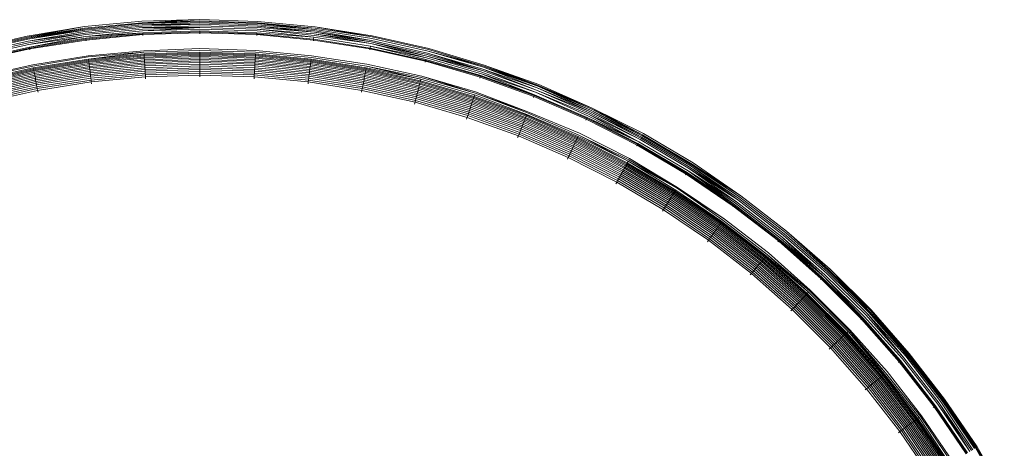
# Model space of a CAD drawing. Units: inches. Extents: x 64 to 1167, y 117 to 939.
# Tile 54 of 56: x 1130.034 to 1131.241, y 501.546 to 502.071. Entities that reach past the tile are written whole.
import ezdxf

# ---------------------------------------------------------------- set-up
doc = ezdxf.new("R2010")
doc.units = ezdxf.units.IN
doc.header["$MEASUREMENT"] = 0
doc.layers.add('A-FLOR-FIXT', color=8, linetype='Continuous', lineweight=18)

msp = doc.modelspace()

# ---------------------------------------------------------------- linework, layer by layer
at = {"layer": 'A-FLOR-FIXT'}
for p, q in [((1130.1137, 502.0626), (1130.0437, 502.0509)), ((1130.1137, 502.0626), (1130.044, 502.0497)), ((1130.1843, 502.0693), (1130.1137, 502.0626)), ((1130.1844, 502.0675), (1130.1139, 502.0608)), ((1130.1845, 502.0663), (1130.114, 502.0596)), ((1130.1845, 502.0649), (1130.1142, 502.0583)), ((1130.1847, 502.0633), (1130.1144, 502.0566)), ((1130.2552, 502.0712), (1130.1843, 502.0693)), ((1130.2552, 502.0712), (1130.1844, 502.0675)), ((1130.2552, 502.0697), (1130.1844, 502.0675)), ((1130.2552, 502.0685), (1130.1844, 502.0675)), ((1130.2552, 502.0685), (1130.1845, 502.0663)), ((1130.2552, 502.0671), (1130.1845, 502.0649)), ((1130.2552, 502.0655), (1130.1845, 502.0649)), ((1130.2552, 502.0655), (1130.1847, 502.0633)), ((1130.2552, 502.0637), (1130.1848, 502.0614)), ((1130.326, 502.0689), (1130.2552, 502.0712)), ((1130.3259, 502.0675), (1130.2552, 502.0697)), ((1130.3258, 502.0663), (1130.2552, 502.0685)), ((1130.3258, 502.0649), (1130.2552, 502.0671)), ((1130.3257, 502.0633), (1130.2552, 502.0655)), ((1130.3255, 502.0614), (1130.2552, 502.0637)), ((1130.396, 502.0575), (1130.3257, 502.0633)), ((1130.3958, 502.0558), (1130.3257, 502.0633)), ((1130.3962, 502.059), (1130.3258, 502.0663)), ((1130.3964, 502.0608), (1130.3258, 502.0663)), ((1130.3962, 502.059), (1130.3258, 502.0649)), ((1130.3964, 502.0608), (1130.3259, 502.0675)), ((1130.3966, 502.0623), (1130.326, 502.0689)), ((1130.0437, 502.0509), (1129.9746, 502.0355)), ((1130.1139, 502.0608), (1130.044, 502.0497)), ((1130.1139, 502.0608), (1130.0442, 502.0486)), ((1130.114, 502.0596), (1130.0442, 502.0486)), ((1130.1142, 502.0583), (1130.0442, 502.0486)), ((1130.1142, 502.0583), (1130.0445, 502.0472)), ((1130.1144, 502.0566), (1130.0449, 502.0447)), ((1130.1147, 502.0548), (1130.0449, 502.0447)), ((1130.1147, 502.0548), (1130.0453, 502.0428)), ((1130.1149, 502.0528), (1130.0457, 502.0408)), ((1130.1152, 502.0507), (1130.0457, 502.0408)), ((1130.1152, 502.0507), (1130.0463, 502.0376)), ((1130.1848, 502.0614), (1130.1147, 502.0548)), ((1130.1849, 502.0595), (1130.1149, 502.0528)), ((1130.185, 502.0573), (1130.1152, 502.0507)), ((1130.1852, 502.0551), (1130.1152, 502.0507)), ((1130.1852, 502.0551), (1130.1155, 502.0485)), ((1130.1852, 502.054), (1130.1156, 502.0474)), ((1130.1853, 502.0528), (1130.1157, 502.0462)), ((1130.2552, 502.0617), (1130.1848, 502.0614)), ((1130.2552, 502.0617), (1130.1849, 502.0595)), ((1130.2552, 502.0617), (1130.185, 502.0573)), ((1130.2552, 502.0595), (1130.185, 502.0573)), ((1130.2552, 502.0573), (1130.1852, 502.0551)), ((1130.2552, 502.0562), (1130.1852, 502.054)), ((1130.1852, 502.054), (1130.1852, 502.0551)), ((1130.1853, 502.0528), (1130.1852, 502.054)), ((1130.2552, 502.055), (1130.1853, 502.0528)), ((1130.1854, 502.0517), (1130.1853, 502.0528)), ((1130.3254, 502.0595), (1130.2552, 502.0617)), ((1130.3253, 502.0573), (1130.2552, 502.0595)), ((1130.3251, 502.0551), (1130.2552, 502.0573)), ((1130.2552, 502.0573), (1130.2552, 502.0562)), ((1130.3251, 502.054), (1130.2552, 502.0562)), ((1130.2552, 502.0562), (1130.2552, 502.055)), ((1130.325, 502.0528), (1130.2552, 502.055)), ((1130.2552, 502.055), (1130.2552, 502.0539)), ((1130.325, 502.0528), (1130.3249, 502.0517)), ((1130.3251, 502.054), (1130.325, 502.0528)), ((1130.3946, 502.0462), (1130.325, 502.0528)), ((1130.3251, 502.0551), (1130.3251, 502.054)), ((1130.395, 502.0496), (1130.3251, 502.0551)), ((1130.3947, 502.0474), (1130.3251, 502.054)), ((1130.395, 502.0496), (1130.3253, 502.0573)), ((1130.3955, 502.0538), (1130.3254, 502.0595)), ((1130.3953, 502.0518), (1130.3254, 502.0595)), ((1130.3958, 502.0558), (1130.3255, 502.0614)), ((1130.4648, 502.0418), (1130.3953, 502.0518)), ((1130.4648, 502.0418), (1130.3955, 502.0538)), ((1130.4652, 502.0438), (1130.3955, 502.0538)), ((1130.4655, 502.0456), (1130.3958, 502.0558)), ((1130.4652, 502.0438), (1130.3958, 502.0558)), ((1130.4655, 502.0456), (1130.396, 502.0575)), ((1130.466, 502.0479), (1130.3962, 502.059)), ((1130.4664, 502.0502), (1130.3964, 502.0608)), ((1130.4666, 502.0514), (1130.3966, 502.0623)), ((1130.4664, 502.0502), (1130.3966, 502.0623)), ((1130.5358, 502.0359), (1130.4666, 502.0514)), ((1130.044, 502.0497), (1129.9749, 502.0343)), ((1130.0442, 502.0486), (1129.9752, 502.0332)), ((1130.0445, 502.0472), (1129.9755, 502.0318)), ((1130.0449, 502.0447), (1129.9761, 502.0294)), ((1130.0453, 502.0428), (1129.9766, 502.0275)), ((1130.0457, 502.0408), (1129.9771, 502.0255)), ((1130.1155, 502.0485), (1130.0463, 502.0376)), ((1130.1156, 502.0474), (1130.0465, 502.0364)), ((1130.1157, 502.0462), (1130.0467, 502.0353)), ((1130.1156, 502.0474), (1130.1155, 502.0485)), ((1130.1157, 502.0462), (1130.1156, 502.0474)), ((1130.1159, 502.0451), (1130.1157, 502.0462)), ((1130.3944, 502.0451), (1130.3946, 502.0462)), ((1130.3946, 502.0462), (1130.3947, 502.0474)), ((1130.4636, 502.0353), (1130.3946, 502.0462)), ((1130.3947, 502.0474), (1130.395, 502.0496)), ((1130.4638, 502.0364), (1130.3947, 502.0474)), ((1130.4642, 502.0387), (1130.395, 502.0496)), ((1130.4642, 502.0387), (1130.4638, 502.0364)), ((1130.5329, 502.0244), (1130.4642, 502.0387)), ((1130.5323, 502.0223), (1130.4642, 502.0387)), ((1130.5329, 502.0244), (1130.4648, 502.0418)), ((1130.5334, 502.0265), (1130.4648, 502.0418)), ((1130.5339, 502.0284), (1130.4652, 502.0438)), ((1130.5334, 502.0265), (1130.4652, 502.0438)), ((1130.5344, 502.0302), (1130.4655, 502.0456)), ((1130.535, 502.0325), (1130.466, 502.0479)), ((1130.5355, 502.0347), (1130.4664, 502.0502)), ((1130.0463, 502.0376), (1129.978, 502.0223)), ((1130.0465, 502.0364), (1129.9782, 502.0212)), ((1130.0467, 502.0353), (1129.9785, 502.0201)), ((1130.0463, 502.0376), (1130.0465, 502.0364)), ((1130.0465, 502.0364), (1130.0467, 502.0353)), ((1130.0467, 502.0353), (1130.0469, 502.0342)), ((1130.1182, 502.0269), (1130.0505, 502.0157)), ((1130.1866, 502.0329), (1130.1182, 502.0269)), ((1130.1867, 502.0314), (1130.1183, 502.0257)), ((1130.1867, 502.0314), (1130.1187, 502.0229)), ((1130.1868, 502.0293), (1130.1187, 502.0229)), ((1130.1869, 502.0281), (1130.1188, 502.0217)), ((1130.1869, 502.0268), (1130.119, 502.0204)), ((1130.2552, 502.0359), (1130.1866, 502.0329)), ((1130.2552, 502.0335), (1130.1867, 502.0314)), ((1130.2552, 502.0315), (1130.1868, 502.0293)), ((1130.1869, 502.0281), (1130.1868, 502.0293)), ((1130.2552, 502.0303), (1130.1869, 502.0281)), ((1130.2552, 502.0289), (1130.1869, 502.0268)), ((1130.1869, 502.0268), (1130.1869, 502.0281)), ((1130.187, 502.0253), (1130.1869, 502.0268)), ((1130.2552, 502.0275), (1130.187, 502.0253)), ((1130.3238, 502.0334), (1130.2552, 502.0359)), ((1130.3236, 502.0314), (1130.2552, 502.0335)), ((1130.3235, 502.0293), (1130.2552, 502.0315)), ((1130.2552, 502.0303), (1130.2552, 502.0315)), ((1130.3234, 502.0281), (1130.2552, 502.0303)), ((1130.2552, 502.0289), (1130.2552, 502.0303)), ((1130.3234, 502.0268), (1130.2552, 502.0289)), ((1130.2552, 502.0275), (1130.2552, 502.0289)), ((1130.3233, 502.0253), (1130.2552, 502.0275)), ((1130.2552, 502.0259), (1130.2552, 502.0275)), ((1130.3233, 502.0253), (1130.3234, 502.0268)), ((1130.3234, 502.0281), (1130.3235, 502.0293)), ((1130.3915, 502.0217), (1130.3234, 502.0281)), ((1130.3234, 502.0268), (1130.3234, 502.0281)), ((1130.3913, 502.0204), (1130.3234, 502.0268)), ((1130.3916, 502.0229), (1130.3235, 502.0293)), ((1130.3919, 502.0249), (1130.3236, 502.0314)), ((1130.3921, 502.0269), (1130.3238, 502.0334)), ((1130.46, 502.0168), (1130.3921, 502.0269)), ((1130.4636, 502.0353), (1130.4634, 502.0342)), ((1130.4638, 502.0364), (1130.4636, 502.0353)), ((1130.5318, 502.0201), (1130.4636, 502.0353)), ((1130.5321, 502.0212), (1130.4638, 502.0364)), ((1130.6009, 502.0069), (1130.5334, 502.0265)), ((1130.6015, 502.0088), (1130.5334, 502.0265)), ((1130.6015, 502.0088), (1130.5339, 502.0284)), ((1130.6015, 502.0088), (1130.5344, 502.0302)), ((1130.6021, 502.0105), (1130.5344, 502.0302)), ((1130.6028, 502.0128), (1130.535, 502.0325)), ((1130.6032, 502.014), (1130.535, 502.0325)), ((1130.6032, 502.014), (1130.5355, 502.0347)), ((1130.6037, 502.0154), (1130.5358, 502.0359)), ((1130.0505, 502.0157), (1129.9834, 502.0012)), ((1130.0507, 502.0142), (1129.9837, 502.0001)), ((1130.1183, 502.0257), (1130.0507, 502.0142)), ((1130.1187, 502.0229), (1130.0511, 502.0122)), ((1130.1188, 502.0217), (1130.0514, 502.011)), ((1130.119, 502.0204), (1130.0516, 502.0097)), ((1130.1192, 502.0189), (1130.0519, 502.0083)), ((1130.1194, 502.0173), (1130.0522, 502.0067)), ((1130.1196, 502.0157), (1130.0525, 502.005)), ((1130.1188, 502.0217), (1130.1187, 502.0229)), ((1130.119, 502.0204), (1130.1188, 502.0217)), ((1130.1192, 502.0189), (1130.119, 502.0204)), ((1130.187, 502.0253), (1130.1192, 502.0189)), ((1130.1194, 502.0173), (1130.1192, 502.0189)), ((1130.1871, 502.0238), (1130.1194, 502.0173)), ((1130.1196, 502.0157), (1130.1194, 502.0173)), ((1130.1872, 502.0221), (1130.1196, 502.0157)), ((1130.1198, 502.0139), (1130.1196, 502.0157)), ((1130.1874, 502.0203), (1130.1198, 502.0139)), ((1130.1875, 502.0184), (1130.1201, 502.012)), ((1130.1876, 502.0165), (1130.1203, 502.0101)), ((1130.1877, 502.0144), (1130.1206, 502.0081)), ((1130.1871, 502.0238), (1130.187, 502.0253)), ((1130.2552, 502.0259), (1130.1871, 502.0238)), ((1130.1872, 502.0221), (1130.1871, 502.0238)), ((1130.2552, 502.0242), (1130.1872, 502.0221)), ((1130.1874, 502.0203), (1130.1872, 502.0221)), ((1130.2552, 502.0224), (1130.1874, 502.0203)), ((1130.1875, 502.0184), (1130.1874, 502.0203)), ((1130.2552, 502.0205), (1130.1875, 502.0184)), ((1130.1876, 502.0165), (1130.1875, 502.0184)), ((1130.2552, 502.0186), (1130.1876, 502.0165)), ((1130.1877, 502.0144), (1130.1876, 502.0165)), ((1130.2552, 502.0165), (1130.1877, 502.0144)), ((1130.1879, 502.0123), (1130.1877, 502.0144)), ((1130.2552, 502.0144), (1130.1879, 502.0123)), ((1130.3232, 502.0238), (1130.2552, 502.0259)), ((1130.2552, 502.0242), (1130.2552, 502.0259)), ((1130.3231, 502.0221), (1130.2552, 502.0242)), ((1130.2552, 502.0224), (1130.2552, 502.0242)), ((1130.2552, 502.0205), (1130.2552, 502.0224)), ((1130.3229, 502.0203), (1130.2552, 502.0224)), ((1130.3228, 502.0184), (1130.2552, 502.0205)), ((1130.2552, 502.0186), (1130.2552, 502.0205)), ((1130.3227, 502.0165), (1130.2552, 502.0186)), ((1130.2552, 502.0165), (1130.2552, 502.0186)), ((1130.3226, 502.0144), (1130.2552, 502.0165)), ((1130.2552, 502.0144), (1130.2552, 502.0165)), ((1130.3224, 502.0123), (1130.2552, 502.0144)), ((1130.2552, 502.0123), (1130.2552, 502.0144)), ((1130.3224, 502.0123), (1130.3226, 502.0144)), ((1130.3226, 502.0144), (1130.3227, 502.0165)), ((1130.3897, 502.0081), (1130.3226, 502.0144)), ((1130.3227, 502.0165), (1130.3228, 502.0184)), ((1130.39, 502.0101), (1130.3227, 502.0165)), ((1130.3228, 502.0184), (1130.3229, 502.0203)), ((1130.3902, 502.012), (1130.3228, 502.0184)), ((1130.3229, 502.0203), (1130.3231, 502.0221)), ((1130.3905, 502.0139), (1130.3229, 502.0203)), ((1130.3231, 502.0221), (1130.3232, 502.0238)), ((1130.3907, 502.0157), (1130.3231, 502.0221)), ((1130.3232, 502.0238), (1130.3233, 502.0253)), ((1130.3909, 502.0173), (1130.3232, 502.0238)), ((1130.3911, 502.0189), (1130.3233, 502.0253)), ((1130.3905, 502.0139), (1130.3907, 502.0157)), ((1130.3907, 502.0157), (1130.3909, 502.0173)), ((1130.4578, 502.005), (1130.3907, 502.0157)), ((1130.3909, 502.0173), (1130.3911, 502.0189)), ((1130.4581, 502.0067), (1130.3909, 502.0173)), ((1130.3911, 502.0189), (1130.3913, 502.0204)), ((1130.4584, 502.0083), (1130.3911, 502.0189)), ((1130.3913, 502.0204), (1130.3915, 502.0217)), ((1130.4587, 502.0097), (1130.3913, 502.0204)), ((1130.3915, 502.0217), (1130.3916, 502.0229)), ((1130.4589, 502.011), (1130.3915, 502.0217)), ((1130.4592, 502.0122), (1130.3916, 502.0229)), ((1130.4596, 502.0142), (1130.3919, 502.0249)), ((1130.5266, 502.0001), (1130.4596, 502.0142)), ((1130.5262, 501.9983), (1130.4596, 502.0142)), ((1130.5271, 502.0018), (1130.46, 502.0168)), ((1130.5315, 502.0189), (1130.5318, 502.0201)), ((1130.5318, 502.0201), (1130.5321, 502.0212)), ((1130.5989, 502.0006), (1130.5318, 502.0201)), ((1130.5321, 502.0212), (1130.5323, 502.0223)), ((1130.5992, 502.0017), (1130.5321, 502.0212)), ((1130.5996, 502.0027), (1130.5323, 502.0223)), ((1130.6003, 502.0049), (1130.5329, 502.0244)), ((1130.6705, 501.9917), (1130.6037, 502.0154)), ((1130.67, 501.9905), (1130.6037, 502.0154)), ((1130.0511, 502.0122), (1129.9844, 501.9973)), ((1130.0514, 502.011), (1129.9847, 501.9961)), ((1130.0516, 502.0097), (1129.985, 501.9948)), ((1130.0519, 502.0083), (1129.9854, 501.9934)), ((1130.0522, 502.0067), (1129.9858, 501.9919)), ((1130.0525, 502.005), (1129.9862, 501.9902)), ((1130.0528, 502.0033), (1129.9866, 501.9885)), ((1130.0514, 502.011), (1130.0511, 502.0122)), ((1130.0516, 502.0097), (1130.0514, 502.011)), ((1130.0519, 502.0083), (1130.0516, 502.0097)), ((1130.0522, 502.0067), (1130.0519, 502.0083)), ((1130.0525, 502.005), (1130.0522, 502.0067)), ((1130.0528, 502.0033), (1130.0525, 502.005)), ((1130.1198, 502.0139), (1130.0528, 502.0033)), ((1130.0532, 502.0014), (1130.0528, 502.0033)), ((1130.1201, 502.012), (1130.0532, 502.0014)), ((1130.1203, 502.0101), (1130.0536, 501.9995)), ((1130.1206, 502.0081), (1130.0539, 501.9975)), ((1130.1208, 502.006), (1130.0543, 501.9955)), ((1130.1211, 502.0038), (1130.0547, 501.9933)), ((1130.1201, 502.012), (1130.1198, 502.0139)), ((1130.1203, 502.0101), (1130.1201, 502.012)), ((1130.1206, 502.0081), (1130.1203, 502.0101)), ((1130.1208, 502.006), (1130.1206, 502.0081)), ((1130.1879, 502.0123), (1130.1208, 502.006)), ((1130.1211, 502.0038), (1130.1208, 502.006)), ((1130.188, 502.0102), (1130.1211, 502.0038)), ((1130.1214, 502.0017), (1130.1211, 502.0038)), ((1130.1881, 502.008), (1130.1214, 502.0017)), ((1130.1883, 502.0057), (1130.1217, 501.9994)), ((1130.1884, 502.0034), (1130.1219, 501.9972)), ((1130.188, 502.0102), (1130.1879, 502.0123)), ((1130.2552, 502.0123), (1130.188, 502.0102)), ((1130.1881, 502.008), (1130.188, 502.0102)), ((1130.2552, 502.0101), (1130.1881, 502.008)), ((1130.1883, 502.0057), (1130.1881, 502.008)), ((1130.2552, 502.0078), (1130.1883, 502.0057)), ((1130.1884, 502.0034), (1130.1883, 502.0057)), ((1130.2552, 502.0055), (1130.1884, 502.0034)), ((1130.1886, 502.0011), (1130.1884, 502.0034)), ((1130.2552, 502.0032), (1130.1886, 502.0011)), ((1130.3223, 502.0102), (1130.2552, 502.0123)), ((1130.2552, 502.0101), (1130.2552, 502.0123)), ((1130.3222, 502.008), (1130.2552, 502.0101)), ((1130.2552, 502.0078), (1130.2552, 502.0101)), ((1130.322, 502.0057), (1130.2552, 502.0078)), ((1130.2552, 502.0055), (1130.2552, 502.0078)), ((1130.3219, 502.0034), (1130.2552, 502.0055)), ((1130.2552, 502.0032), (1130.2552, 502.0055)), ((1130.3217, 502.0011), (1130.2552, 502.0032)), ((1130.2552, 502.0009), (1130.2552, 502.0032)), ((1130.3217, 502.0011), (1130.3219, 502.0034)), ((1130.3219, 502.0034), (1130.322, 502.0057)), ((1130.3884, 501.9972), (1130.3219, 502.0034)), ((1130.322, 502.0057), (1130.3222, 502.008)), ((1130.3886, 501.9994), (1130.322, 502.0057)), ((1130.3222, 502.008), (1130.3223, 502.0102)), ((1130.3889, 502.0017), (1130.3222, 502.008)), ((1130.3223, 502.0102), (1130.3224, 502.0123)), ((1130.3892, 502.0038), (1130.3223, 502.0102)), ((1130.3895, 502.006), (1130.3224, 502.0123)), ((1130.3889, 502.0017), (1130.3892, 502.0038)), ((1130.3892, 502.0038), (1130.3895, 502.006)), ((1130.4556, 501.9933), (1130.3892, 502.0038)), ((1130.3895, 502.006), (1130.3897, 502.0081)), ((1130.456, 501.9955), (1130.3895, 502.006)), ((1130.3897, 502.0081), (1130.39, 502.0101)), ((1130.4564, 501.9975), (1130.3897, 502.0081)), ((1130.39, 502.0101), (1130.3902, 502.012)), ((1130.4567, 501.9995), (1130.39, 502.0101)), ((1130.3902, 502.012), (1130.3905, 502.0139)), ((1130.4571, 502.0014), (1130.3902, 502.012)), ((1130.4575, 502.0033), (1130.3905, 502.0139)), ((1130.4571, 502.0014), (1130.4575, 502.0033)), ((1130.4575, 502.0033), (1130.4578, 502.005)), ((1130.5237, 501.9885), (1130.4575, 502.0033)), ((1130.4578, 502.005), (1130.4581, 502.0067)), ((1130.5241, 501.9902), (1130.4578, 502.005)), ((1130.4581, 502.0067), (1130.4584, 502.0083)), ((1130.5245, 501.9919), (1130.4581, 502.0067)), ((1130.4584, 502.0083), (1130.4587, 502.0097)), ((1130.5249, 501.9934), (1130.4584, 502.0083)), ((1130.4587, 502.0097), (1130.4589, 502.011)), ((1130.5253, 501.9948), (1130.4587, 502.0097)), ((1130.4589, 502.011), (1130.4592, 502.0122)), ((1130.5256, 501.9961), (1130.4589, 502.011)), ((1130.5262, 501.9983), (1130.4592, 502.0122)), ((1130.5992, 502.0017), (1130.5996, 502.0027)), ((1130.6655, 501.979), (1130.5996, 502.0027)), ((1130.6655, 501.979), (1130.6003, 502.0049)), ((1130.6667, 501.9821), (1130.6003, 502.0049)), ((1130.6667, 501.9821), (1130.6009, 502.0069)), ((1130.6678, 501.9849), (1130.6015, 502.0088)), ((1130.6678, 501.9849), (1130.6021, 502.0105)), ((1130.6688, 501.9874), (1130.6021, 502.0105)), ((1130.6688, 501.9874), (1130.6028, 502.0128)), ((1130.6696, 501.9895), (1130.6028, 502.0128)), ((1130.67, 501.9905), (1130.6032, 502.014)), ((1130.6696, 501.9895), (1130.6032, 502.014)), ((1130.0532, 502.0014), (1129.9871, 501.9867)), ((1130.0536, 501.9995), (1129.9876, 501.9848)), ((1130.0539, 501.9975), (1129.9881, 501.9828)), ((1130.0543, 501.9955), (1129.9886, 501.9808)), ((1130.0547, 501.9933), (1129.9892, 501.9787)), ((1130.0551, 501.9912), (1129.9897, 501.9765)), ((1130.0536, 501.9995), (1130.0532, 502.0014)), ((1130.0539, 501.9975), (1130.0536, 501.9995)), ((1130.0543, 501.9955), (1130.0539, 501.9975)), ((1130.0547, 501.9933), (1130.0543, 501.9955)), ((1130.0551, 501.9912), (1130.0547, 501.9933)), ((1130.1214, 502.0017), (1130.0551, 501.9912)), ((1130.0556, 501.989), (1130.0551, 501.9912)), ((1130.1217, 501.9994), (1130.0556, 501.989)), ((1130.1219, 501.9972), (1130.056, 501.9867)), ((1130.1222, 501.9949), (1130.0564, 501.9845)), ((1130.1217, 501.9994), (1130.1214, 502.0017)), ((1130.1219, 501.9972), (1130.1217, 501.9994)), ((1130.1222, 501.9949), (1130.1219, 501.9972)), ((1130.1886, 502.0011), (1130.1222, 501.9949)), ((1130.1225, 501.9926), (1130.1222, 501.9949)), ((1130.1887, 501.9988), (1130.1886, 502.0011)), ((1130.3216, 501.9988), (1130.3217, 502.0011)), ((1130.3881, 501.9949), (1130.3217, 502.0011)), ((1130.3878, 501.9926), (1130.3881, 501.9949)), ((1130.3881, 501.9949), (1130.3884, 501.9972)), ((1130.4539, 501.9845), (1130.3881, 501.9949)), ((1130.3884, 501.9972), (1130.3886, 501.9994)), ((1130.4543, 501.9867), (1130.3884, 501.9972)), ((1130.3886, 501.9994), (1130.3889, 502.0017)), ((1130.4547, 501.989), (1130.3886, 501.9994)), ((1130.4552, 501.9912), (1130.3889, 502.0017)), ((1130.4552, 501.9912), (1130.4547, 501.989)), ((1130.4552, 501.9912), (1130.4556, 501.9933)), ((1130.5206, 501.9765), (1130.4552, 501.9912)), ((1130.4556, 501.9933), (1130.456, 501.9955)), ((1130.5211, 501.9787), (1130.4556, 501.9933)), ((1130.456, 501.9955), (1130.4564, 501.9975)), ((1130.5217, 501.9808), (1130.456, 501.9955)), ((1130.4564, 501.9975), (1130.4567, 501.9995)), ((1130.5222, 501.9828), (1130.4564, 501.9975)), ((1130.4567, 501.9995), (1130.4571, 502.0014)), ((1130.5227, 501.9848), (1130.4567, 501.9995)), ((1130.5232, 501.9867), (1130.4571, 502.0014)), ((1130.5241, 501.9902), (1130.5237, 501.9885)), ((1130.5245, 501.9919), (1130.5241, 501.9902)), ((1130.5894, 501.9713), (1130.5241, 501.9902)), ((1130.5249, 501.9934), (1130.5245, 501.9919)), ((1130.5899, 501.9729), (1130.5245, 501.9919)), ((1130.5253, 501.9948), (1130.5249, 501.9934)), ((1130.5904, 501.9744), (1130.5249, 501.9934)), ((1130.5256, 501.9961), (1130.5253, 501.9948)), ((1130.5908, 501.9758), (1130.5253, 501.9948)), ((1130.5262, 501.9983), (1130.5256, 501.9961)), ((1130.5912, 501.977), (1130.5256, 501.9961)), ((1130.5919, 501.9792), (1130.5262, 501.9983)), ((1130.5925, 501.9809), (1130.5266, 502.0001)), ((1130.5925, 501.9809), (1130.5271, 502.0018)), ((1130.593, 501.9826), (1130.5271, 502.0018)), ((1130.5985, 501.9995), (1130.5989, 502.0006)), ((1130.5992, 502.0017), (1130.5989, 502.0006)), ((1130.6646, 501.9769), (1130.5989, 502.0006)), ((1130.665, 501.978), (1130.5992, 502.0017)), ((1130.7354, 501.9632), (1130.67, 501.9905)), ((1130.7348, 501.9619), (1130.67, 501.9905)), ((1130.7354, 501.9632), (1130.6705, 501.9917)), ((1130.0556, 501.989), (1129.9903, 501.9744)), ((1130.056, 501.9867), (1129.9908, 501.9721)), ((1130.0564, 501.9845), (1129.9914, 501.9699)), ((1130.056, 501.9867), (1130.0556, 501.989)), ((1130.0564, 501.9845), (1130.056, 501.9867)), ((1130.0569, 501.9822), (1130.0564, 501.9845)), ((1130.4539, 501.9845), (1130.4534, 501.9822)), ((1130.4543, 501.9867), (1130.4539, 501.9845)), ((1130.5189, 501.9699), (1130.4539, 501.9845)), ((1130.4547, 501.989), (1130.4543, 501.9867)), ((1130.5195, 501.9721), (1130.4543, 501.9867)), ((1130.52, 501.9744), (1130.4547, 501.989)), ((1130.5211, 501.9787), (1130.5206, 501.9765)), ((1130.5217, 501.9808), (1130.5211, 501.9787)), ((1130.5857, 501.9599), (1130.5211, 501.9787)), ((1130.5222, 501.9828), (1130.5217, 501.9808)), ((1130.5863, 501.962), (1130.5217, 501.9808)), ((1130.5227, 501.9848), (1130.5222, 501.9828)), ((1130.587, 501.964), (1130.5222, 501.9828)), ((1130.5232, 501.9867), (1130.5227, 501.9848)), ((1130.5876, 501.9659), (1130.5227, 501.9848)), ((1130.5237, 501.9885), (1130.5232, 501.9867)), ((1130.5882, 501.9678), (1130.5232, 501.9867)), ((1130.5888, 501.9696), (1130.5237, 501.9885)), ((1130.5919, 501.9792), (1130.5912, 501.977)), ((1130.656, 501.955), (1130.5919, 501.9792)), ((1130.6573, 501.9583), (1130.5925, 501.9809)), ((1130.6567, 501.9569), (1130.5925, 501.9809)), ((1130.6573, 501.9583), (1130.593, 501.9826)), ((1130.6646, 501.9769), (1130.665, 501.978)), ((1130.665, 501.978), (1130.6655, 501.979)), ((1130.7292, 501.9502), (1130.665, 501.978)), ((1130.7297, 501.9512), (1130.6655, 501.979)), ((1130.7316, 501.9552), (1130.6667, 501.9821)), ((1130.7307, 501.9532), (1130.6667, 501.9821)), ((1130.7324, 501.957), (1130.6678, 501.9849)), ((1130.7332, 501.9586), (1130.6678, 501.9849)), ((1130.7332, 501.9586), (1130.6688, 501.9874)), ((1130.7339, 501.9601), (1130.6688, 501.9874)), ((1130.7339, 501.9601), (1130.6696, 501.9895)), ((1130.7348, 501.9619), (1130.6696, 501.9895)), ((1130.5183, 501.9677), (1130.5189, 501.9699)), ((1130.5189, 501.9699), (1130.5195, 501.9721)), ((1130.5829, 501.9513), (1130.5189, 501.9699)), ((1130.5195, 501.9721), (1130.52, 501.9744)), ((1130.5836, 501.9535), (1130.5195, 501.9721)), ((1130.52, 501.9744), (1130.5206, 501.9765)), ((1130.5843, 501.9557), (1130.52, 501.9744)), ((1130.585, 501.9578), (1130.5206, 501.9765)), ((1130.5876, 501.9659), (1130.587, 501.964)), ((1130.5882, 501.9678), (1130.5876, 501.9659)), ((1130.6512, 501.943), (1130.5876, 501.9659)), ((1130.5888, 501.9696), (1130.5882, 501.9678)), ((1130.6519, 501.9449), (1130.5882, 501.9678)), ((1130.5894, 501.9713), (1130.5888, 501.9696)), ((1130.6526, 501.9466), (1130.5888, 501.9696)), ((1130.5899, 501.9729), (1130.5894, 501.9713)), ((1130.6533, 501.9483), (1130.5894, 501.9713)), ((1130.5904, 501.9744), (1130.5899, 501.9729)), ((1130.6539, 501.9498), (1130.5899, 501.9729)), ((1130.5908, 501.9758), (1130.5904, 501.9744)), ((1130.6545, 501.9513), (1130.5904, 501.9744)), ((1130.5912, 501.977), (1130.5908, 501.9758)), ((1130.655, 501.9527), (1130.5908, 501.9758)), ((1130.6555, 501.9539), (1130.5912, 501.977)), ((1130.6642, 501.9758), (1130.6646, 501.9769)), ((1130.7287, 501.9491), (1130.6646, 501.9769)), ((1130.5843, 501.9557), (1130.5836, 501.9535)), ((1130.585, 501.9578), (1130.5843, 501.9557)), ((1130.6472, 501.933), (1130.5843, 501.9557)), ((1130.5857, 501.9599), (1130.585, 501.9578)), ((1130.6481, 501.9351), (1130.585, 501.9578)), ((1130.5863, 501.962), (1130.5857, 501.9599)), ((1130.6489, 501.9372), (1130.5857, 501.9599)), ((1130.587, 501.964), (1130.5863, 501.962)), ((1130.6497, 501.9392), (1130.5863, 501.962)), ((1130.6505, 501.9411), (1130.587, 501.964)), ((1130.655, 501.9527), (1130.6555, 501.9539)), ((1130.6555, 501.9539), (1130.656, 501.955)), ((1130.7182, 501.9268), (1130.6555, 501.9539)), ((1130.7187, 501.9279), (1130.656, 501.955)), ((1130.7196, 501.9297), (1130.6567, 501.9569)), ((1130.7206, 501.9319), (1130.6573, 501.9583)), ((1130.7947, 501.9241), (1130.7316, 501.9552)), ((1130.7932, 501.9214), (1130.7316, 501.9552)), ((1130.7947, 501.9241), (1130.7324, 501.957)), ((1130.7965, 501.9273), (1130.7332, 501.9586)), ((1130.7956, 501.9258), (1130.7332, 501.9586)), ((1130.7965, 501.9273), (1130.7339, 501.9601)), ((1130.7972, 501.9287), (1130.7339, 501.9601)), ((1130.7972, 501.9287), (1130.7348, 501.9619)), ((1130.7978, 501.9298), (1130.7348, 501.9619)), ((1130.7988, 501.9316), (1130.7354, 501.9632)), ((1130.7978, 501.9298), (1130.7354, 501.9632)), ((1130.5829, 501.9513), (1130.5822, 501.9491)), ((1130.5836, 501.9535), (1130.5829, 501.9513)), ((1130.6456, 501.9288), (1130.5829, 501.9513)), ((1130.6464, 501.9309), (1130.5836, 501.9535)), ((1130.6505, 501.9411), (1130.6512, 501.943)), ((1130.6512, 501.943), (1130.6519, 501.9449)), ((1130.7132, 501.9162), (1130.6512, 501.943)), ((1130.6519, 501.9449), (1130.6526, 501.9466)), ((1130.7141, 501.918), (1130.6519, 501.9449)), ((1130.6526, 501.9466), (1130.6533, 501.9483)), ((1130.7149, 501.9197), (1130.6526, 501.9466)), ((1130.6533, 501.9483), (1130.6539, 501.9498)), ((1130.7156, 501.9213), (1130.6533, 501.9483)), ((1130.6539, 501.9498), (1130.6545, 501.9513)), ((1130.7163, 501.9228), (1130.6539, 501.9498)), ((1130.6545, 501.9513), (1130.655, 501.9527)), ((1130.717, 501.9242), (1130.6545, 501.9513)), ((1130.7176, 501.9256), (1130.655, 501.9527)), ((1130.7287, 501.9491), (1130.7283, 501.9481)), ((1130.7292, 501.9502), (1130.7287, 501.9491)), ((1130.791, 501.9174), (1130.7287, 501.9491)), ((1130.7297, 501.9512), (1130.7292, 501.9502)), ((1130.7916, 501.9184), (1130.7292, 501.9502)), ((1130.7921, 501.9194), (1130.7297, 501.9512)), ((1130.7932, 501.9214), (1130.7297, 501.9512)), ((1130.7932, 501.9214), (1130.7307, 501.9532)), ((1130.6456, 501.9288), (1130.6464, 501.9309)), ((1130.6464, 501.9309), (1130.6472, 501.933)), ((1130.7077, 501.9044), (1130.6464, 501.9309)), ((1130.6472, 501.933), (1130.6481, 501.9351)), ((1130.7087, 501.9064), (1130.6472, 501.933)), ((1130.6481, 501.9351), (1130.6489, 501.9372)), ((1130.7096, 501.9085), (1130.6481, 501.9351)), ((1130.6489, 501.9372), (1130.6497, 501.9392)), ((1130.7106, 501.9105), (1130.6489, 501.9372)), ((1130.6497, 501.9392), (1130.6505, 501.9411)), ((1130.7115, 501.9124), (1130.6497, 501.9392)), ((1130.7124, 501.9143), (1130.6505, 501.9411)), ((1130.7802, 501.8978), (1130.7196, 501.9297)), ((1130.7811, 501.8993), (1130.7196, 501.9297)), ((1130.7819, 501.9009), (1130.7206, 501.9319)), ((1130.8587, 501.8938), (1130.7978, 501.9298)), ((1130.8598, 501.8955), (1130.7988, 501.9316)), ((1130.6447, 501.9266), (1130.6456, 501.9288)), ((1130.7067, 501.9023), (1130.6456, 501.9288)), ((1130.7132, 501.9162), (1130.7141, 501.918)), ((1130.7141, 501.918), (1130.7149, 501.9197)), ((1130.7744, 501.8872), (1130.7141, 501.918)), ((1130.7149, 501.9197), (1130.7156, 501.9213)), ((1130.7753, 501.8889), (1130.7149, 501.9197)), ((1130.7156, 501.9213), (1130.7163, 501.9228)), ((1130.7762, 501.8904), (1130.7156, 501.9213)), ((1130.7163, 501.9228), (1130.717, 501.9242)), ((1130.777, 501.8919), (1130.7163, 501.9228)), ((1130.717, 501.9242), (1130.7176, 501.9256)), ((1130.7777, 501.8933), (1130.717, 501.9242)), ((1130.7176, 501.9256), (1130.7182, 501.9268)), ((1130.7784, 501.8946), (1130.7176, 501.9256)), ((1130.7182, 501.9268), (1130.7187, 501.9279)), ((1130.7791, 501.8958), (1130.7182, 501.9268)), ((1130.7802, 501.8978), (1130.7187, 501.9279)), ((1130.791, 501.9174), (1130.7916, 501.9184)), ((1130.7916, 501.9184), (1130.7921, 501.9194)), ((1130.8518, 501.8828), (1130.7916, 501.9184)), ((1130.8524, 501.8838), (1130.7921, 501.9194)), ((1130.8536, 501.8857), (1130.7932, 501.9214)), ((1130.8553, 501.8883), (1130.7947, 501.9241)), ((1130.8563, 501.8899), (1130.7956, 501.9258)), ((1130.8572, 501.8914), (1130.7965, 501.9273)), ((1130.858, 501.8927), (1130.7972, 501.9287)), ((1130.7077, 501.9044), (1130.7087, 501.9064)), ((1130.7087, 501.9064), (1130.7096, 501.9085)), ((1130.7683, 501.8761), (1130.7087, 501.9064)), ((1130.7096, 501.9085), (1130.7106, 501.9105)), ((1130.7694, 501.878), (1130.7096, 501.9085)), ((1130.7106, 501.9105), (1130.7115, 501.9124)), ((1130.7704, 501.88), (1130.7106, 501.9105)), ((1130.7115, 501.9124), (1130.7124, 501.9143)), ((1130.7715, 501.8819), (1130.7115, 501.9124)), ((1130.7124, 501.9143), (1130.7132, 501.9162)), ((1130.7725, 501.8837), (1130.7124, 501.9143)), ((1130.7735, 501.8855), (1130.7132, 501.9162)), ((1130.7904, 501.9164), (1130.791, 501.9174)), ((1130.8512, 501.8819), (1130.791, 501.9174)), ((1130.7057, 501.9002), (1130.7067, 501.9023)), ((1130.7067, 501.9023), (1130.7077, 501.9044)), ((1130.7661, 501.8721), (1130.7067, 501.9023)), ((1130.7672, 501.8741), (1130.7077, 501.9044)), ((1130.7784, 501.8946), (1130.7777, 501.8933)), ((1130.7791, 501.8958), (1130.7784, 501.8946)), ((1130.8372, 501.8598), (1130.7784, 501.8946)), ((1130.7802, 501.8978), (1130.7791, 501.8958)), ((1130.8379, 501.861), (1130.7791, 501.8958)), ((1130.8386, 501.862), (1130.7802, 501.8978)), ((1130.8401, 501.8644), (1130.7802, 501.8978)), ((1130.8401, 501.8644), (1130.7811, 501.8993)), ((1130.8407, 501.8654), (1130.7819, 501.9009)), ((1130.8401, 501.8644), (1130.7819, 501.9009)), ((1130.9169, 501.8535), (1130.8587, 501.8938)), ((1130.9181, 501.8552), (1130.8587, 501.8938)), ((1130.9181, 501.8552), (1130.8598, 501.8955)), ((1130.7715, 501.8819), (1130.7704, 501.88)), ((1130.7725, 501.8837), (1130.7715, 501.8819)), ((1130.8294, 501.8476), (1130.7715, 501.8819)), ((1130.7735, 501.8855), (1130.7725, 501.8837)), ((1130.8305, 501.8494), (1130.7725, 501.8837)), ((1130.7744, 501.8872), (1130.7735, 501.8855)), ((1130.8316, 501.8511), (1130.7735, 501.8855)), ((1130.7753, 501.8889), (1130.7744, 501.8872)), ((1130.8327, 501.8528), (1130.7744, 501.8872)), ((1130.7762, 501.8904), (1130.7753, 501.8889)), ((1130.8337, 501.8543), (1130.7753, 501.8889)), ((1130.777, 501.8919), (1130.7762, 501.8904)), ((1130.8346, 501.8558), (1130.7762, 501.8904)), ((1130.7777, 501.8933), (1130.777, 501.8919)), ((1130.8355, 501.8573), (1130.777, 501.8919)), ((1130.8364, 501.8586), (1130.7777, 501.8933)), ((1130.8512, 501.8819), (1130.8505, 501.8809)), ((1130.8518, 501.8828), (1130.8512, 501.8819)), ((1130.9089, 501.8426), (1130.8512, 501.8819)), ((1130.8524, 501.8838), (1130.8518, 501.8828)), ((1130.9096, 501.8435), (1130.8518, 501.8828)), ((1130.9103, 501.8444), (1130.8524, 501.8838)), ((1130.9116, 501.8462), (1130.8536, 501.8857)), ((1130.9129, 501.848), (1130.8536, 501.8857)), ((1130.9103, 501.8444), (1130.8536, 501.8857)), ((1130.9129, 501.848), (1130.8553, 501.8883)), ((1130.9146, 501.8503), (1130.8553, 501.8883)), ((1130.9146, 501.8503), (1130.8563, 501.8899)), ((1130.9156, 501.8517), (1130.8572, 501.8914)), ((1130.9146, 501.8503), (1130.8572, 501.8914)), ((1130.9169, 501.8535), (1130.858, 501.8927)), ((1130.7661, 501.8721), (1130.765, 501.87)), ((1130.7672, 501.8741), (1130.7661, 501.8721)), ((1130.8234, 501.8381), (1130.7661, 501.8721)), ((1130.7683, 501.8761), (1130.7672, 501.8741)), ((1130.8246, 501.8401), (1130.7672, 501.8741)), ((1130.7694, 501.878), (1130.7683, 501.8761)), ((1130.8259, 501.842), (1130.7683, 501.8761)), ((1130.7704, 501.88), (1130.7694, 501.878)), ((1130.8271, 501.8439), (1130.7694, 501.878)), ((1130.8283, 501.8458), (1130.7704, 501.88)), ((1130.8346, 501.8558), (1130.8355, 501.8573)), ((1130.8355, 501.8573), (1130.8364, 501.8586)), ((1130.8918, 501.819), (1130.8355, 501.8573)), ((1130.8364, 501.8586), (1130.8372, 501.8598)), ((1130.8928, 501.8203), (1130.8364, 501.8586)), ((1130.8372, 501.8598), (1130.8379, 501.861)), ((1130.8936, 501.8215), (1130.8372, 501.8598)), ((1130.8379, 501.861), (1130.8386, 501.862)), ((1130.8944, 501.8226), (1130.8379, 501.861)), ((1130.8951, 501.8236), (1130.8386, 501.862)), ((1130.8963, 501.8252), (1130.8401, 501.8644)), ((1130.8977, 501.8271), (1130.8401, 501.8644)), ((1130.8977, 501.8271), (1130.8407, 501.8654)), ((1130.8271, 501.8439), (1130.8283, 501.8458)), ((1130.8283, 501.8458), (1130.8294, 501.8476)), ((1130.8838, 501.808), (1130.8283, 501.8458)), ((1130.8294, 501.8476), (1130.8305, 501.8494)), ((1130.8851, 501.8098), (1130.8294, 501.8476)), ((1130.8305, 501.8494), (1130.8316, 501.8511)), ((1130.8863, 501.8115), (1130.8305, 501.8494)), ((1130.8316, 501.8511), (1130.8327, 501.8528)), ((1130.8875, 501.8131), (1130.8316, 501.8511)), ((1130.8327, 501.8528), (1130.8337, 501.8543)), ((1130.8887, 501.8147), (1130.8327, 501.8528)), ((1130.8337, 501.8543), (1130.8346, 501.8558)), ((1130.8898, 501.8162), (1130.8337, 501.8543)), ((1130.8908, 501.8177), (1130.8346, 501.8558)), ((1130.967, 501.8032), (1130.9116, 501.8462)), ((1130.9684, 501.8049), (1130.9129, 501.848)), ((1130.9703, 501.8071), (1130.9146, 501.8503)), ((1130.9714, 501.8085), (1130.9156, 501.8517)), ((1130.9728, 501.8102), (1130.9169, 501.8535)), ((1130.9741, 501.8117), (1130.9181, 501.8552)), ((1130.8222, 501.8362), (1130.8234, 501.8381)), ((1130.8234, 501.8381), (1130.8246, 501.8401)), ((1130.8785, 501.8007), (1130.8234, 501.8381)), ((1130.8246, 501.8401), (1130.8259, 501.842)), ((1130.8799, 501.8026), (1130.8246, 501.8401)), ((1130.8259, 501.842), (1130.8271, 501.8439)), ((1130.8812, 501.8044), (1130.8259, 501.842)), ((1130.8825, 501.8062), (1130.8271, 501.8439)), ((1130.9089, 501.8426), (1130.9083, 501.8416)), ((1130.9089, 501.8426), (1130.9096, 501.8435)), ((1130.9642, 501.7998), (1130.9089, 501.8426)), ((1130.9096, 501.8435), (1130.9103, 501.8444)), ((1130.9649, 501.8006), (1130.9096, 501.8435)), ((1130.9656, 501.8015), (1130.9103, 501.8444)), ((1130.8928, 501.8203), (1130.8936, 501.8215)), ((1130.8936, 501.8215), (1130.8944, 501.8226)), ((1130.9475, 501.7797), (1130.8936, 501.8215)), ((1130.8944, 501.8226), (1130.8951, 501.8236)), ((1130.9484, 501.7807), (1130.8944, 501.8226)), ((1130.9492, 501.7816), (1130.8951, 501.8236)), ((1130.9505, 501.7832), (1130.8963, 501.8252)), ((1130.9521, 501.7852), (1130.8977, 501.8271)), ((1130.8838, 501.808), (1130.8851, 501.8098)), ((1130.8851, 501.8098), (1130.8863, 501.8115)), ((1130.9383, 501.7685), (1130.8851, 501.8098)), ((1130.8863, 501.8115), (1130.8875, 501.8131)), ((1130.9396, 501.7701), (1130.8863, 501.8115)), ((1130.8875, 501.8131), (1130.8887, 501.8147)), ((1130.9409, 501.7717), (1130.8875, 501.8131)), ((1130.8887, 501.8147), (1130.8898, 501.8162)), ((1130.9422, 501.7732), (1130.8887, 501.8147)), ((1130.8898, 501.8162), (1130.8908, 501.8177)), ((1130.9434, 501.7746), (1130.8898, 501.8162)), ((1130.8908, 501.8177), (1130.8918, 501.819)), ((1130.9445, 501.776), (1130.8908, 501.8177)), ((1130.8918, 501.819), (1130.8928, 501.8203)), ((1130.9456, 501.7773), (1130.8918, 501.819)), ((1130.9466, 501.7785), (1130.8928, 501.8203)), ((1131.0258, 501.7634), (1130.9728, 501.8102)), ((1131.0276, 501.7653), (1130.9741, 501.8117)), ((1131.0266, 501.7642), (1130.9741, 501.8117)), ((1130.8772, 501.7988), (1130.8785, 501.8007)), ((1130.8785, 501.8007), (1130.8799, 501.8026)), ((1130.9312, 501.7599), (1130.8785, 501.8007)), ((1130.8799, 501.8026), (1130.8812, 501.8044)), ((1130.9326, 501.7616), (1130.8799, 501.8026)), ((1130.8812, 501.8044), (1130.8825, 501.8062)), ((1130.9341, 501.7634), (1130.8812, 501.8044)), ((1130.8825, 501.8062), (1130.8838, 501.808)), ((1130.9355, 501.7651), (1130.8825, 501.8062)), ((1130.9369, 501.7668), (1130.8838, 501.808)), ((1130.9634, 501.7989), (1130.9642, 501.7998)), ((1130.9642, 501.7998), (1130.9649, 501.8006)), ((1131.0166, 501.7535), (1130.9642, 501.7998)), ((1130.9649, 501.8006), (1130.9656, 501.8015)), ((1131.0174, 501.7544), (1130.9649, 501.8006)), ((1131.0181, 501.7552), (1130.9656, 501.8015)), ((1131.0197, 501.7568), (1130.9656, 501.8015)), ((1131.0197, 501.7568), (1130.967, 501.8032)), ((1131.0197, 501.7568), (1130.9684, 501.8049)), ((1131.0211, 501.7584), (1130.9684, 501.8049)), ((1131.0231, 501.7605), (1130.9703, 501.8071)), ((1131.0243, 501.7618), (1130.9714, 501.8085)), ((1131.0033, 501.7394), (1130.9521, 501.7852)), ((1130.9422, 501.7732), (1130.9409, 501.7717)), ((1130.9434, 501.7746), (1130.9422, 501.7732)), ((1130.993, 501.7284), (1130.9422, 501.7732)), ((1130.9445, 501.776), (1130.9434, 501.7746)), ((1130.9943, 501.7298), (1130.9434, 501.7746)), ((1130.9456, 501.7773), (1130.9445, 501.776)), ((1130.9955, 501.7311), (1130.9445, 501.776)), ((1130.9466, 501.7785), (1130.9456, 501.7773)), ((1130.9966, 501.7323), (1130.9456, 501.7773)), ((1130.9475, 501.7797), (1130.9466, 501.7785)), ((1130.9977, 501.7335), (1130.9466, 501.7785)), ((1130.9484, 501.7807), (1130.9475, 501.7797)), ((1130.9987, 501.7345), (1130.9475, 501.7797)), ((1130.9492, 501.7816), (1130.9484, 501.7807)), ((1130.9996, 501.7355), (1130.9484, 501.7807)), ((1131.0012, 501.7372), (1130.9492, 501.7816)), ((1131.0012, 501.7372), (1130.9505, 501.7832)), ((1131.0024, 501.7385), (1130.9505, 501.7832)), ((1130.9326, 501.7616), (1130.9312, 501.7599)), ((1130.9341, 501.7634), (1130.9326, 501.7616)), ((1130.9827, 501.7175), (1130.9326, 501.7616)), ((1130.9355, 501.7651), (1130.9341, 501.7634)), ((1130.9843, 501.7191), (1130.9341, 501.7634)), ((1130.9369, 501.7668), (1130.9355, 501.7651)), ((1130.9858, 501.7208), (1130.9355, 501.7651)), ((1130.9383, 501.7685), (1130.9369, 501.7668)), ((1130.9873, 501.7224), (1130.9369, 501.7668)), ((1130.9396, 501.7701), (1130.9383, 501.7685)), ((1130.9888, 501.724), (1130.9383, 501.7685)), ((1130.9409, 501.7717), (1130.9396, 501.7701)), ((1130.9902, 501.7255), (1130.9396, 501.7701)), ((1130.9916, 501.727), (1130.9409, 501.7717)), ((1131.0748, 501.7124), (1131.0243, 501.7618)), ((1131.0758, 501.7134), (1131.0258, 501.7634)), ((1131.077, 501.7145), (1131.0258, 501.7634)), ((1131.077, 501.7145), (1131.0266, 501.7642)), ((1131.078, 501.7154), (1131.0276, 501.7653)), ((1131.077, 501.7145), (1131.0276, 501.7653)), ((1130.9297, 501.7581), (1130.9312, 501.7599)), ((1130.9811, 501.7158), (1130.9312, 501.7599)), ((1131.0166, 501.7535), (1131.0158, 501.7527)), ((1131.0174, 501.7544), (1131.0166, 501.7535)), ((1131.066, 501.7041), (1131.0166, 501.7535)), ((1131.0181, 501.7552), (1131.0174, 501.7544)), ((1131.0668, 501.7049), (1131.0174, 501.7544)), ((1131.0677, 501.7057), (1131.0181, 501.7552)), ((1131.0693, 501.7072), (1131.0197, 501.7568)), ((1131.0677, 501.7057), (1131.0197, 501.7568)), ((1131.0716, 501.7094), (1131.0211, 501.7584)), ((1131.073, 501.7107), (1131.0231, 501.7605)), ((1131.0012, 501.7372), (1130.9996, 501.7355)), ((1131.0496, 501.6888), (1131.0012, 501.7372)), ((1131.0509, 501.69), (1131.0024, 501.7385)), ((1131.0518, 501.6908), (1131.0033, 501.7394)), ((1130.9902, 501.7255), (1130.9888, 501.724)), ((1130.9916, 501.727), (1130.9902, 501.7255)), ((1131.0379, 501.6778), (1130.9902, 501.7255)), ((1130.993, 501.7284), (1130.9916, 501.727)), ((1131.0394, 501.6792), (1130.9916, 501.727)), ((1130.9943, 501.7298), (1130.993, 501.7284)), ((1131.0409, 501.6805), (1130.993, 501.7284)), ((1130.9955, 501.7311), (1130.9943, 501.7298)), ((1131.0422, 501.6818), (1130.9943, 501.7298)), ((1130.9966, 501.7323), (1130.9955, 501.7311)), ((1131.0435, 501.683), (1130.9955, 501.7311)), ((1130.9977, 501.7335), (1130.9966, 501.7323)), ((1131.0448, 501.6842), (1130.9966, 501.7323)), ((1130.9987, 501.7345), (1130.9977, 501.7335)), ((1131.0459, 501.6853), (1130.9977, 501.7335)), ((1130.9996, 501.7355), (1130.9987, 501.7345)), ((1131.047, 501.6863), (1130.9987, 501.7345)), ((1131.048, 501.6872), (1130.9996, 501.7355)), ((1130.9811, 501.7158), (1130.9796, 501.7141)), ((1130.9827, 501.7175), (1130.9811, 501.7158)), ((1131.0282, 501.6687), (1130.9811, 501.7158)), ((1130.9843, 501.7191), (1130.9827, 501.7175)), ((1131.0299, 501.6703), (1130.9827, 501.7175)), ((1130.9858, 501.7208), (1130.9843, 501.7191)), ((1131.0316, 501.6718), (1130.9843, 501.7191)), ((1130.9873, 501.7224), (1130.9858, 501.7208)), ((1131.0332, 501.6734), (1130.9858, 501.7208)), ((1130.9888, 501.724), (1130.9873, 501.7224)), ((1131.0348, 501.6749), (1130.9873, 501.7224)), ((1131.0364, 501.6764), (1130.9888, 501.724)), ((1131.1226, 501.6603), (1131.0758, 501.7134)), ((1131.1244, 501.6618), (1131.077, 501.7145)), ((1131.1226, 501.6603), (1131.077, 501.7145)), ((1131.1235, 501.6611), (1131.077, 501.7145)), ((1131.1244, 501.6618), (1131.078, 501.7154)), ((1131.066, 501.7041), (1131.0651, 501.7033)), ((1131.0668, 501.7049), (1131.066, 501.7041)), ((1131.1122, 501.6517), (1131.066, 501.7041)), ((1131.0677, 501.7057), (1131.0668, 501.7049)), ((1131.1131, 501.6524), (1131.0668, 501.7049)), ((1131.114, 501.6532), (1131.0677, 501.7057)), ((1131.1165, 501.6553), (1131.0693, 501.7072)), ((1131.1181, 501.6566), (1131.0716, 501.7094)), ((1131.1203, 501.6584), (1131.073, 501.7107)), ((1131.1181, 501.6566), (1131.073, 501.7107)), ((1131.1215, 501.6594), (1131.0748, 501.7124)), ((1131.048, 501.6872), (1131.0496, 501.6888)), ((1131.0941, 501.6367), (1131.0496, 501.6888)), ((1131.0957, 501.638), (1131.0496, 501.6888)), ((1131.0957, 501.638), (1131.0509, 501.69)), ((1131.0977, 501.6397), (1131.0518, 501.6908)), ((1131.0348, 501.6749), (1131.0364, 501.6764)), ((1131.0364, 501.6764), (1131.0379, 501.6778)), ((1131.0809, 501.6259), (1131.0364, 501.6764)), ((1131.0379, 501.6778), (1131.0394, 501.6792)), ((1131.0826, 501.6272), (1131.0379, 501.6778)), ((1131.0394, 501.6792), (1131.0409, 501.6805)), ((1131.0841, 501.6285), (1131.0394, 501.6792)), ((1131.0409, 501.6805), (1131.0422, 501.6818)), ((1131.0856, 501.6297), (1131.0409, 501.6805)), ((1131.0422, 501.6818), (1131.0435, 501.683)), ((1131.0871, 501.6309), (1131.0422, 501.6818)), ((1131.0435, 501.683), (1131.0448, 501.6842)), ((1131.0885, 501.6321), (1131.0435, 501.683)), ((1131.0448, 501.6842), (1131.0459, 501.6853)), ((1131.0898, 501.6332), (1131.0448, 501.6842)), ((1131.0459, 501.6853), (1131.047, 501.6863)), ((1131.091, 501.6342), (1131.0459, 501.6853)), ((1131.047, 501.6863), (1131.048, 501.6872)), ((1131.0921, 501.6351), (1131.047, 501.6863)), ((1131.0931, 501.636), (1131.048, 501.6872)), ((1131.0266, 501.6671), (1131.0282, 501.6687)), ((1131.0282, 501.6687), (1131.0299, 501.6703)), ((1131.0723, 501.6187), (1131.0282, 501.6687)), ((1131.0299, 501.6703), (1131.0316, 501.6718)), ((1131.0741, 501.6202), (1131.0299, 501.6703)), ((1131.0316, 501.6718), (1131.0332, 501.6734)), ((1131.0758, 501.6216), (1131.0316, 501.6718)), ((1131.0332, 501.6734), (1131.0348, 501.6749)), ((1131.0776, 501.6231), (1131.0332, 501.6734)), ((1131.0793, 501.6245), (1131.0348, 501.6749)), ((1131.1122, 501.6517), (1131.1131, 501.6524)), ((1131.1131, 501.6524), (1131.114, 501.6532)), ((1131.156, 501.5972), (1131.1131, 501.6524)), ((1131.1569, 501.5978), (1131.114, 501.6532)), ((1131.1596, 501.5998), (1131.1165, 501.6553)), ((1131.1612, 501.601), (1131.1181, 501.6566)), ((1131.1635, 501.6027), (1131.1203, 501.6584)), ((1131.1648, 501.6036), (1131.1215, 501.6594)), ((1131.166, 501.6044), (1131.1226, 501.6603)), ((1131.1669, 501.6051), (1131.1235, 501.6611)), ((1131.1679, 501.6058), (1131.1244, 501.6618)), ((1131.1113, 501.651), (1131.1122, 501.6517)), ((1131.155, 501.5965), (1131.1122, 501.6517)), ((1131.0826, 501.6272), (1131.0841, 501.6285)), ((1131.0841, 501.6285), (1131.0856, 501.6297)), ((1131.1255, 501.5751), (1131.0841, 501.6285)), ((1131.0856, 501.6297), (1131.0871, 501.6309)), ((1131.1271, 501.5762), (1131.0856, 501.6297)), ((1131.0871, 501.6309), (1131.0885, 501.6321)), ((1131.1287, 501.5773), (1131.0871, 501.6309)), ((1131.0885, 501.6321), (1131.0898, 501.6332)), ((1131.1301, 501.5784), (1131.0885, 501.6321)), ((1131.0898, 501.6332), (1131.091, 501.6342)), ((1131.1315, 501.5794), (1131.0898, 501.6332)), ((1131.091, 501.6342), (1131.0921, 501.6351)), ((1131.1327, 501.5803), (1131.091, 501.6342)), ((1131.0921, 501.6351), (1131.0931, 501.636)), ((1131.1339, 501.5812), (1131.0921, 501.6351)), ((1131.0931, 501.636), (1131.0941, 501.6367)), ((1131.135, 501.582), (1131.0931, 501.636)), ((1131.1369, 501.5833), (1131.0941, 501.6367)), ((1131.1383, 501.5844), (1131.0957, 501.638)), ((1131.1398, 501.5854), (1131.0977, 501.6397)), ((1131.0705, 501.6172), (1131.0723, 501.6187)), ((1131.0723, 501.6187), (1131.0741, 501.6202)), ((1131.1131, 501.5661), (1131.0723, 501.6187)), ((1131.0741, 501.6202), (1131.0758, 501.6216)), ((1131.115, 501.5674), (1131.0741, 501.6202)), ((1131.0758, 501.6216), (1131.0776, 501.6231)), ((1131.1168, 501.5688), (1131.0758, 501.6216)), ((1131.0776, 501.6231), (1131.0793, 501.6245)), ((1131.1187, 501.5701), (1131.0776, 501.6231)), ((1131.0793, 501.6245), (1131.0809, 501.6259)), ((1131.1205, 501.5714), (1131.0793, 501.6245)), ((1131.0809, 501.6259), (1131.0826, 501.6272)), ((1131.1222, 501.5727), (1131.0809, 501.6259)), ((1131.1239, 501.5739), (1131.0826, 501.6272)), ((1131.2057, 501.546), (1131.166, 501.6044)), ((1131.2067, 501.5466), (1131.166, 501.6044)), ((1131.2067, 501.5466), (1131.1669, 501.6051)), ((1131.2067, 501.5466), (1131.1679, 501.6058)), ((1131.2077, 501.5472), (1131.1679, 501.6058)), ((1131.1541, 501.5958), (1131.155, 501.5965)), ((1131.155, 501.5965), (1131.156, 501.5972)), ((1131.1943, 501.5387), (1131.155, 501.5965)), ((1131.156, 501.5972), (1131.1569, 501.5978)), ((1131.1953, 501.5393), (1131.156, 501.5972)), ((1131.1962, 501.5399), (1131.1569, 501.5978)), ((1131.199, 501.5417), (1131.1596, 501.5998)), ((1131.199, 501.5417), (1131.1612, 501.601)), ((1131.2008, 501.5428), (1131.1612, 501.601)), ((1131.2024, 501.5438), (1131.1635, 501.6027)), ((1131.2045, 501.5452), (1131.1648, 501.6036)), ((1131.2057, 501.546), (1131.1648, 501.6036)), ((1131.1315, 501.5794), (1131.1327, 501.5803)), ((1131.1327, 501.5803), (1131.1339, 501.5812)), ((1131.171, 501.524), (1131.1327, 501.5803)), ((1131.1339, 501.5812), (1131.135, 501.582)), ((1131.1723, 501.5247), (1131.1339, 501.5812)), ((1131.135, 501.582), (1131.1369, 501.5833)), ((1131.1734, 501.5255), (1131.135, 501.582)), ((1131.1744, 501.5261), (1131.1369, 501.5833)), ((1131.1769, 501.5276), (1131.1383, 501.5844)), ((1131.1784, 501.5286), (1131.1398, 501.5854)), ((1131.115, 501.5674), (1131.1168, 501.5688)), ((1131.1168, 501.5688), (1131.1187, 501.5701)), ((1131.1545, 501.5134), (1131.1168, 501.5688)), ((1131.1187, 501.5701), (1131.1205, 501.5714)), ((1131.1564, 501.5146), (1131.1187, 501.5701)), ((1131.1205, 501.5714), (1131.1222, 501.5727)), ((1131.1582, 501.5158), (1131.1205, 501.5714)), ((1131.1222, 501.5727), (1131.1239, 501.5739)), ((1131.16, 501.517), (1131.1222, 501.5727)), ((1131.1239, 501.5739), (1131.1255, 501.5751)), ((1131.1618, 501.5181), (1131.1239, 501.5739)), ((1131.1255, 501.5751), (1131.1271, 501.5762)), ((1131.1635, 501.5192), (1131.1255, 501.5751)), ((1131.1271, 501.5762), (1131.1287, 501.5773)), ((1131.1652, 501.5202), (1131.1271, 501.5762)), ((1131.1287, 501.5773), (1131.1301, 501.5784)), ((1131.1668, 501.5212), (1131.1287, 501.5773)), ((1131.1301, 501.5784), (1131.1315, 501.5794)), ((1131.1683, 501.5222), (1131.1301, 501.5784)), ((1131.1697, 501.5231), (1131.1315, 501.5794)), ((1131.1113, 501.5647), (1131.1131, 501.5661)), ((1131.1131, 501.5661), (1131.115, 501.5674)), ((1131.1506, 501.511), (1131.1131, 501.5661)), ((1131.1525, 501.5122), (1131.115, 501.5674)), ((1131.2411, 501.4848), (1131.2057, 501.546)), ((1131.2248, 501.5176), (1131.2067, 501.5466)), ((1131.2248, 501.5176), (1131.2077, 501.5472))]:
    msp.add_line(p, q, dxfattribs=at)

doc.saveas('drawing.dxf')
